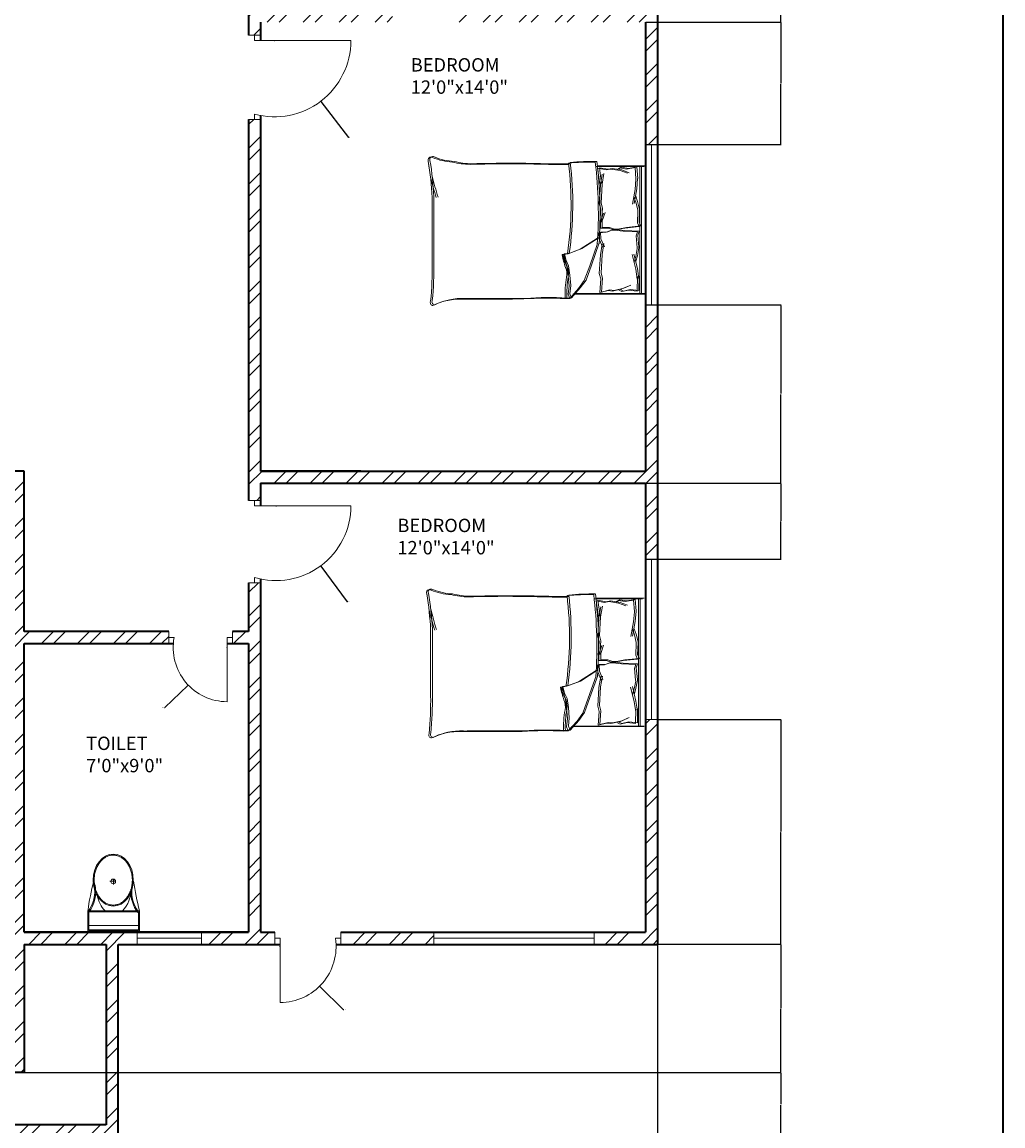
# Model space of a CAD drawing. Units: inches. Extents: x 392 to 1254, y 1207 to 2665.
# Tile 4 of 15: x 887 to 1254, y 1414 to 1827. Entities that reach past the tile are written whole.
import ezdxf

# ---------------------------------------------------------------- set-up
doc = ezdxf.new("R2010")
doc.units = ezdxf.units.IN
for name, color, linetype, lineweight in [('A-ANNO-DIMS', 2, 'Continuous', 18), ('A-ANNO-TTLB', 7, 'Continuous', 35), ('A-AREA-IDEN', 7, 'Continuous', 18), ('A-DOOR', 3, 'Continuous', 18), ('A-FLOR-FIXT', 9, 'Continuous', 18), ('A-FURN', 8, 'Continuous', 13), ('A-GLAZ', 4, 'Continuous', 18), ('A-WALL', 7, 'Continuous', 35), ('A-WALL-PATT', 252, 'Continuous', 13)]:
    doc.layers.add(name, color=color, linetype=linetype, lineweight=lineweight)
doc.styles.get("Standard").update_dxf_attribs({"font": 'arial.ttf'})
doc.dimstyles.get("Standard").update_dxf_attribs({"dimtxt": 0.18, "dimasz": 0.18, "dimexe": 0.18, "dimexo": 0.0625, "dimgap": 0.09, "dimtad": 0, "dimtih": 1, "dimtoh": 1, "dimdec": 4, "dimzin": 0, "dimdsep": 46, "dimtxsty": 'Standard', "dimcen": 0.09, "dimadec": 0, "dimazin": 0, "dimtfac": 1, "dimtdec": 4, "dimtofl": 0, "dimtmove": 0, "dimatfit": 3, "dimfxl": 1, "dimtolj": 1, "dimtzin": 0, "dimarcsym": 0})

# ---------------------------------------------------------------- blocks, each defined once
blk = doc.blocks.new('A$C31115884')
for p, q in [((283, 498), (223, 498)), ((258, 466), (258, 523)), ((0, 200), (0, 0)), ((520, 200), (0, 200)), ((10, 190), (10, 10)), ((510, 190), (10, 190)), ((510, 10), (510, 190)), ((520, 0), (520, 200)), ((510, 54), (0, 54)), ((10, 10), (510, 10)), ((0, 0), (520, 0))]:
    blk.add_line(p, q)
blk.add_circle((256, 496), 23.6)
for centre, radius, start, end in [((2778, -205), 2807, 165.4549, 171.7133), ((-295, 403), 365, 324.2091, 9.3499), ((-295, 403), 375, 324.2091, 9.3499), ((806, 403), 365, 170.6501, 215.7909), ((3237, 905), 2807, 188.2867, 194.5451), ((384, 406), 293, 190.2774, 224.1564), ((139, 406), 293, 315.8436, 2.6563), ((806, 403), 375, 179.2036, 215.7909)]:
    blk.add_arc(centre, radius, start, end)
blk.add_ellipse((256, 510), major_axis=(0, -261), ratio=0.772727)
blk.add_open_spline([(256, 259), (263, 259), (270, 260), (288, 262), (299, 265), (320, 273), (330, 278), (350, 291), (360, 299), (378, 316), (386, 326), (402, 347), (409, 358), (421, 383), (427, 395), (436, 422), (440, 436), (445, 465), (447, 480), (448, 509), (448, 524), (445, 553), (443, 568), (436, 596), (432, 610), (422, 636), (416, 649), (402, 672), (395, 683), (379, 703), (370, 712), (351, 728), (341, 735), (321, 746), (310, 751), (289, 757), (278, 759), (256, 761), (245, 761), (223, 757), (212, 754), (191, 746), (181, 741), (161, 728), (151, 720), (133, 703), (125, 693), (110, 672), (103, 660), (90, 636), (85, 623), (76, 596), (72, 582), (67, 553), (66, 538), (64, 509), (65, 494), (68, 465), (70, 450), (77, 422), (81, 408), (91, 382), (97, 370), (111, 346), (118, 335), (135, 316), (144, 307), (162, 291), (172, 284), (193, 273), (203, 269), (225, 262), (236, 260), (250, 259), (253, 259), (256, 259)], degree=3, knots=[0, 0, 0, 0, 0.110105, 0.110105, 0.285049, 0.285049, 0.459994, 0.459994, 0.634938, 0.634938, 0.809882, 0.809882, 0.984827, 0.984827, 1.159771, 1.159771, 1.334715, 1.334715, 1.50966, 1.50966, 1.684604, 1.684604, 1.859549, 1.859549, 2.034493, 2.034493, 2.209437, 2.209437, 2.384382, 2.384382, 2.559326, 2.559326, 2.73427, 2.73427, 2.909215, 2.909215, 3.084159, 3.084159, 3.259103, 3.259103, 3.434048, 3.434048, 3.608992, 3.608992, 3.783936, 3.783936, 3.958881, 3.958881, 4.133825, 4.133825, 4.30877, 4.30877, 4.483714, 4.483714, 4.658658, 4.658658, 4.833603, 4.833603, 5.008547, 5.008547, 5.183491, 5.183491, 5.358436, 5.358436, 5.53338, 5.53338, 5.708324, 5.708324, 5.883269, 5.883269, 6.058213, 6.058213, 6.233158, 6.233158, 6.283185, 6.283185, 6.283185, 6.283185])
blk = doc.blocks.new('BED-DOUBLE')
for p, q in [((3.47, 63.33), (3.47, 81.44)), ((3.47, 79.91), (51.27, 79.91)), ((3.48, 63.33), (3.48, 81.44)), ((3.48, 79.91), (51.27, 79.91)), ((3.7, 62.69), (3.7, 80.8)), ((3.7, 62.69), (3.7, 80.8)), ((3.7, 79.27), (51.49, 79.27)), ((3.7, 79.27), (51.49, 79.27)), ((16.88, 78.42), (19.77, 79.14)), ((16.88, 78.42), (19.77, 79.14)), ((17.11, 77.78), (20, 78.5)), ((17.11, 77.78), (20, 78.5)), ((19.77, 79.14), (20.09, 79.14)), ((19.77, 79.14), (20.09, 79.14)), ((20, 78.5), (20.32, 78.5)), ((20, 78.5), (20.32, 78.5)), ((20.09, 79.14), (24.54, 78.99)), ((20.09, 79.14), (24.54, 78.99)), ((20.32, 78.5), (24.77, 78.35)), ((20.32, 78.5), (24.77, 78.35)), ((24.54, 78.99), (25.98, 79.57)), ((24.54, 78.99), (25.98, 79.57)), ((24.77, 78.35), (26.21, 78.93)), ((24.77, 78.35), (26.21, 78.93)), ((25.98, 79.57), (26.56, 74.22)), ((25.98, 79.57), (26.56, 74.22)), ((26.21, 78.93), (26.79, 73.58)), ((26.21, 78.93), (26.79, 73.58)), ((27.98, 78.95), (27.73, 73.58)), ((27.98, 78.95), (27.73, 73.58)), ((29.46, 78.46), (27.98, 78.95)), ((29.46, 78.46), (27.98, 78.95)), ((33.88, 78.89), (29.46, 78.46)), ((33.88, 78.89), (29.46, 78.46)), ((34.2, 78.91), (33.88, 78.89)), ((34.2, 78.91), (33.88, 78.89)), ((37.14, 78.36), (34.2, 78.91)), ((37.14, 78.36), (34.2, 78.91)), ((45.71, 78.9), (41.91, 78.37)), ((45.71, 78.9), (41.91, 78.37)), ((50.11, 78.89), (44.71, 78.98)), ((44.71, 78.98), (45.71, 78.9)), ((50.11, 78.89), (44.71, 78.98)), ((44.71, 78.98), (45.71, 78.9)), ((50.11, 78.89), (49.73, 75.67)), ((50.11, 78.89), (49.73, 75.67)), ((51.27, 81.44), (51.27, 54.83)), ((51.27, 81.44), (51.27, 54.83)), ((51.49, 81.44), (51.49, 80.8)), ((51.49, 80.8), (51.49, 54.19)), ((51.49, 80.8), (51.49, 54.19)), ((3.89, 78.13), (4.47, 74.95)), ((3.89, 78.13), (4.47, 74.95)), ((3.9, 78.1), (8.18, 78.43)), ((3.9, 78.1), (8.18, 78.43)), ((4.47, 74.95), (4.04, 72.34)), ((4.47, 74.95), (4.04, 72.34)), ((4.12, 77.49), (4.7, 74.31)), ((4.12, 77.49), (4.7, 74.31)), ((4.13, 77.47), (8.41, 77.79)), ((4.13, 77.47), (8.41, 77.79)), ((5.05, 72.49), (6.06, 75.23)), ((5.05, 72.49), (6.06, 75.23)), ((5.28, 71.85), (6.29, 74.6)), ((5.28, 71.85), (6.29, 74.6)), ((8.18, 78.43), (8.28, 78.42)), ((8.18, 78.43), (8.28, 78.42)), ((8.28, 78.42), (12.11, 78.13)), ((8.28, 78.42), (12.11, 78.13)), ((8.41, 77.79), (8.51, 77.78)), ((8.41, 77.79), (8.51, 77.78)), ((8.51, 77.78), (12.34, 77.49)), ((8.51, 77.78), (12.34, 77.49)), ((12.11, 78.13), (17.6, 77.11)), ((12.11, 78.13), (17.6, 77.11)), ((12.34, 77.49), (17.83, 76.48)), ((12.34, 77.49), (17.83, 76.48)), ((14.85, 77.69), (16.88, 78.42)), ((14.85, 77.69), (16.88, 78.42)), ((15.08, 77.05), (17.11, 77.78)), ((15.08, 77.05), (17.11, 77.78)), ((28.21, 78.31), (27.96, 72.94)), ((28.21, 78.31), (27.96, 72.94)), ((29.68, 77.82), (28.21, 78.31)), ((29.68, 77.82), (28.21, 78.31)), ((34.11, 78.25), (29.68, 77.82)), ((34.11, 78.25), (29.68, 77.82)), ((34.43, 78.27), (34.11, 78.25)), ((34.43, 78.27), (34.11, 78.25)), ((37.36, 77.73), (34.43, 78.27)), ((37.36, 77.73), (34.43, 78.27)), ((41.91, 78.37), (36.49, 77.02)), ((41.91, 78.37), (36.5, 77.02)), ((42.14, 77.73), (36.72, 76.38)), ((42.14, 77.73), (36.72, 76.38)), ((39.2, 77.77), (37.14, 78.36)), ((39.2, 77.77), (37.14, 78.36)), ((39.43, 77.13), (37.36, 77.73)), ((39.43, 77.13), (37.36, 77.73)), ((45.94, 78.26), (42.14, 77.73)), ((45.94, 78.26), (42.14, 77.73)), ((50.34, 78.25), (44.94, 78.34)), ((44.94, 78.34), (45.94, 78.26)), ((50.34, 78.25), (44.94, 78.34)), ((44.94, 78.34), (45.94, 78.26)), ((49.31, 73.19), (48.13, 75.86)), ((49.31, 73.19), (48.13, 75.86)), ((49.54, 72.55), (48.36, 75.22)), ((49.54, 72.55), (48.36, 75.22)), ((49.73, 75.67), (50.33, 73.1)), ((49.73, 75.67), (50.33, 73.1)), ((50.34, 78.25), (49.96, 75.04)), ((50.34, 78.25), (49.96, 75.04)), ((49.96, 75.04), (50.56, 72.47)), ((49.96, 75.04), (50.56, 72.47)), ((4.04, 72.34), (4.62, 71.33)), ((4.04, 72.34), (4.62, 71.33)), ((4.7, 74.31), (4.27, 71.7)), ((4.7, 74.31), (4.27, 71.7)), ((4.27, 71.7), (4.85, 70.69)), ((4.27, 71.7), (4.85, 70.69)), ((4.47, 68.87), (5.05, 72.49)), ((4.47, 68.87), (5.05, 72.49)), ((4.7, 68.23), (5.28, 71.85)), ((4.7, 68.23), (5.28, 71.85)), ((26.56, 74.22), (27.14, 71.04)), ((26.56, 74.22), (27.14, 71.04)), ((26.79, 73.58), (27.37, 70.4)), ((26.79, 73.58), (27.37, 70.4)), ((27.14, 71.04), (27.14, 69.74)), ((27.14, 71.04), (27.14, 69.74)), ((27.73, 73.58), (27.35, 70.36)), ((27.73, 73.58), (27.35, 70.36)), ((27.35, 70.36), (27.44, 69.07)), ((27.35, 70.36), (27.44, 69.07)), ((27.37, 70.4), (27.37, 69.1)), ((27.37, 70.4), (27.37, 69.1)), ((27.96, 72.94), (27.58, 69.73)), ((27.96, 72.94), (27.58, 69.73)), ((50.11, 69.61), (49.31, 73.19)), ((50.11, 69.61), (49.31, 73.19)), ((50.34, 68.97), (49.54, 72.55)), ((50.34, 68.97), (49.54, 72.55)), ((50.33, 73.1), (49.81, 72.06)), ((50.33, 73.1), (49.81, 72.06)), ((50.56, 72.47), (50.04, 71.42)), ((50.56, 72.47), (50.04, 71.42)), ((4.18, 64.1), (4.76, 67.28)), ((4.18, 64.1), (4.76, 67.28)), ((4.41, 63.46), (4.99, 66.64)), ((4.41, 63.46), (4.99, 66.64)), ((4.76, 67.28), (4.47, 68.87)), ((4.76, 67.28), (4.47, 68.87)), ((4.99, 66.64), (4.7, 68.23)), ((4.99, 66.64), (4.7, 68.23)), ((24.1, 65.18), (20.96, 66.27)), ((24.1, 65.18), (20.96, 66.27)), ((27.14, 69.74), (26.56, 67.86)), ((27.14, 69.74), (26.56, 67.86)), ((26.56, 67.86), (26.56, 65.18)), ((26.56, 67.86), (26.56, 65.18)), ((27.37, 69.1), (26.79, 67.22)), ((27.37, 69.1), (26.79, 67.22)), ((26.79, 67.22), (26.79, 64.54)), ((26.79, 67.22), (26.79, 64.54)), ((27.44, 69.07), (28.13, 67.23)), ((27.44, 69.07), (28.13, 67.23)), ((27.58, 69.73), (27.66, 68.43)), ((27.58, 69.73), (27.66, 68.43)), ((27.66, 68.43), (28.36, 66.59)), ((27.66, 68.43), (28.36, 66.59)), ((28.13, 67.23), (28.3, 64.55)), ((28.13, 67.23), (28.3, 64.55)), ((28.36, 66.59), (28.53, 63.91)), ((28.36, 66.59), (28.53, 63.91)), ((49.92, 68.01), (50.11, 69.61)), ((49.92, 68.01), (50.11, 69.61)), ((50.7, 64.87), (49.92, 68.01)), ((50.7, 64.87), (49.92, 68.01)), ((50.15, 67.37), (50.34, 68.97)), ((50.15, 67.37), (50.34, 68.97)), ((50.93, 64.23), (50.15, 67.37)), ((50.93, 64.23), (50.15, 67.37)), ((9.28, 64.82), (4.18, 64.1)), ((9.28, 64.82), (4.18, 64.1)), ((9.51, 64.19), (4.41, 63.46)), ((9.51, 64.19), (4.41, 63.46)), ((6.38, 65.81), (10.41, 65.15)), ((6.38, 65.81), (10.41, 65.15)), ((6.61, 65.17), (10.64, 64.51)), ((6.61, 65.17), (10.64, 64.51)), ((10.41, 65.15), (9.28, 64.82)), ((10.41, 65.15), (9.28, 64.82)), ((10.64, 64.51), (9.51, 64.19)), ((10.64, 64.51), (9.51, 64.19)), ((10.41, 65.15), (17.42, 64.72)), ((10.41, 65.15), (17.42, 64.72)), ((10.64, 64.51), (17.65, 64.08)), ((10.64, 64.51), (17.65, 64.08)), ((17.42, 64.72), (19.38, 65.27)), ((17.42, 64.72), (19.38, 65.27)), ((17.65, 64.08), (19.61, 64.63)), ((17.65, 64.08), (19.61, 64.63)), ((19.38, 65.27), (24.52, 64.87)), ((19.38, 65.27), (24.52, 64.87)), ((19.61, 64.63), (24.74, 64.23)), ((19.61, 64.63), (24.74, 64.23)), ((24.33, 64.54), (21.19, 65.63)), ((24.33, 64.54), (21.19, 65.63)), ((26.56, 65.18), (24.1, 65.18)), ((26.56, 65.18), (24.1, 65.18)), ((26.79, 64.54), (24.33, 64.54)), ((26.79, 64.54), (24.33, 64.54)), ((28.3, 64.55), (30.75, 64.7)), ((28.3, 64.55), (30.75, 64.7)), ((28.53, 63.91), (30.98, 64.06)), ((28.53, 63.91), (30.98, 64.06)), ((30.26, 64.06), (34.45, 57.57)), ((30.26, 64.06), (34.45, 57.57)), ((30.49, 63.42), (34.68, 56.93)), ((30.49, 63.42), (34.68, 56.93)), ((30.75, 64.7), (33.82, 65.99)), ((30.75, 64.7), (33.82, 65.99)), ((30.98, 64.06), (34.05, 65.35)), ((30.98, 64.06), (34.05, 65.35)), ((40.64, 61.13), (32.31, 64.06)), ((40.64, 61.13), (32.31, 64.06)), ((40.87, 60.49), (32.53, 63.42)), ((40.87, 60.49), (32.53, 63.42)), ((32.56, 65.81), (36.6, 65.15)), ((32.56, 65.81), (36.6, 65.15)), ((32.79, 65.17), (36.82, 64.51)), ((32.79, 65.17), (36.82, 64.51)), ((36.6, 65.15), (43.61, 64.72)), ((36.6, 65.15), (43.61, 64.72)), ((36.82, 64.51), (43.83, 64.08)), ((36.82, 64.51), (43.83, 64.08)), ((43.61, 64.72), (45.57, 65.27)), ((43.61, 64.72), (45.57, 65.27)), ((43.83, 64.08), (45.79, 64.63)), ((43.83, 64.08), (45.79, 64.63)), ((45.57, 65.27), (50.7, 64.87)), ((45.57, 65.27), (50.7, 64.87)), ((45.79, 64.63), (50.93, 64.23)), ((45.79, 64.63), (50.93, 64.23)), ((46.22, 59.11), (40.64, 61.13)), ((46.22, 59.11), (40.64, 61.13)), ((46.45, 58.47), (40.87, 60.49)), ((46.45, 58.47), (40.87, 60.49)), ((49.16, 56.95), (46.22, 59.11)), ((49.16, 56.95), (46.22, 59.11)), ((49.39, 56.31), (46.45, 58.47)), ((49.39, 56.31), (46.45, 58.47)), ((34.45, 57.57), (36.15, 53.08)), ((34.45, 57.57), (36.15, 53.08)), ((34.68, 56.93), (36.38, 52.44)), ((34.68, 56.93), (36.38, 52.44)), ((52.87, 53.7), (49.16, 56.95)), ((52.87, 53.7), (49.16, 56.95)), ((53.1, 53.06), (49.39, 56.31)), ((53.1, 53.06), (49.39, 56.31)), ((51.33, 53.08), (52.87, 53.7)), ((51.33, 53.08), (52.87, 53.7)), ((52.95, 51.95), (52.87, 53.7, 3.87)), ((52.95, 51.95), (52.87, 53.7, 3.87)), ((36.15, 53.08), (36.46, 51.07)), ((36.15, 53.08), (36.46, 51.07)), ((36.38, 52.44), (36.69, 50.43)), ((36.38, 52.44), (36.69, 50.43)), ((36.46, 51.07), (38.94, 51.68)), ((36.46, 51.07), (38.94, 51.68)), ((36.69, 50.43), (39.17, 51.05)), ((36.69, 50.43), (39.17, 51.05)), ((38.94, 51.68), (40.95, 52.61)), ((38.94, 51.68), (40.95, 52.61)), ((39.17, 51.05), (41.18, 51.97)), ((39.17, 51.05), (41.18, 51.97)), ((40.95, 52.61), (44.36, 53.08)), ((40.95, 52.61), (44.36, 53.08)), ((41.18, 51.97), (44.59, 52.44)), ((41.18, 51.97), (44.59, 52.44)), ((44.36, 53.08), (48.23, 53.39)), ((44.36, 53.08), (48.23, 53.39)), ((44.59, 52.44), (48.46, 52.75)), ((44.59, 52.44), (48.46, 52.75)), ((48.23, 53.39), (51.33, 53.08)), ((48.23, 53.39), (51.33, 53.08)), ((48.46, 52.75), (51.56, 52.44)), ((48.46, 52.75), (51.56, 52.44)), ((51.56, 52.44), (53.1, 53.06)), ((51.56, 52.44), (53.1, 53.06)), ((53.18, 51.31), (53.1, 53.06, 3.87)), ((53.18, 51.31), (53.1, 53.06, 3.87)), ((15.06, 2.2), (39.68, 2.2)), ((15.06, 2.2), (39.68, 2.2)), ((15.29, 1.56), (39.91, 1.56)), ((15.29, 1.56), (39.91, 1.56))]:
    blk.add_line(p, q)
for centre, radius, start, end in [((85.16, 61.35), 83.31, 178.7218, 185.604), ((85.16, 61.35), 83.31, 178.7218, 185.604), ((21.36, -100.61), 164.97, 86.0865, 96.7821), ((21.36, -100.61), 164.97, 86.0865, 96.7821), ((85.39, 60.71), 83.31, 178.7218, 185.604), ((85.39, 60.71), 83.31, 178.7218, 185.604), ((21.59, -101.25), 164.97, 86.0865, 96.7821), ((21.59, -101.25), 164.97, 86.0865, 96.7821), ((17.76, -74.87), 129.02, 81.7845, 96.9006), ((17.76, -74.87), 129.02, 81.7845, 96.9006), ((17.98, -75.51), 129.02, 81.7845, 96.9006), ((17.98, -75.51), 129.02, 81.7845, 96.9006), ((-167.31, 50.27), 170.11, 358.4762, 1.0082), ((-167.31, 50.27), 170.11, 358.4762, 1.0082), ((-167.08, 49.63), 170.11, 358.4762, 1.0082), ((-167.08, 49.63), 170.11, 358.4762, 1.0082), ((36.64, 51), 0.185, 160.2464, 271.1377), ((36.64, 51), 0.185, 160.2464, 271.1377), ((31.15, 79.96), 29.65, 280.6617, 289.8806), ((31.15, 79.96), 29.65, 280.6617, 289.8806), ((36.86, 50.36), 0.185, 160.2464, 271.1377), ((36.86, 50.36), 0.185, 160.2464, 271.1377), ((31.38, 79.32), 29.65, 280.6617, 289.8806), ((31.38, 79.32), 29.65, 280.6617, 289.8806), ((43.74, 46.38), 6.22, 78.6608, 113.7384), ((43.74, 46.38), 6.22, 78.6608, 113.7384), ((43.97, 45.74), 6.22, 78.6608, 113.7384), ((43.97, 45.74), 6.22, 78.6608, 113.7384), ((51.33, 88.1), 36.18, 259.8763, 272.5657), ((51.33, 88.1), 36.18, 259.8763, 272.5657), ((51.56, 87.46), 36.18, 259.8763, 272.5657), ((51.56, 87.46), 36.18, 259.8763, 272.5657), ((182.27, 45.13), 129.5, 176.9791, 183.8365), ((182.27, 45.13), 129.5, 176.9791, 183.8365), ((182.49, 44.49), 129.5, 176.9791, 183.8365), ((182.49, 44.49), 129.5, 176.9791, 183.8365), ((484.82, 30.83), 482.31, 178.2277, 181.7185), ((484.82, 30.83), 482.31, 178.2277, 181.7185), ((485.05, 30.19), 482.31, 178.2277, 181.7185), ((485.05, 30.19), 482.31, 178.2277, 181.7185), ((-4508.74, 13.62), 4561.86, 0.00217, 0.28689), ((-4508.74, 13.62), 4561.86, 0.00217, 0.28689), ((-4508.51, 12.98), 4561.86, 0.00217, 0.28689), ((-4508.52, 12.98), 4561.86, 0.00217, 0.28689), ((-26.9, 16.93), 29.63, 346.0648, 358.9113), ((-26.9, 16.93), 29.63, 346.0648, 358.9113), ((-26.67, 16.29), 29.63, 346.0648, 358.9113), ((-26.67, 16.29), 29.63, 346.0648, 358.9113), ((76.16, 12.78), 23.07, 177.4714, 206.4681), ((76.16, 12.78), 23.07, 177.4714, 206.4681), ((76.39, 12.14), 23.07, 177.4714, 206.4681), ((76.39, 12.14), 23.07, 177.4714, 206.4681), ((-21.66, 11.17), 23.56, 337.9751, 356.652), ((-21.66, 11.17), 23.56, 337.9751, 356.652), ((-21.43, 10.53), 23.56, 337.9751, 356.652), ((-21.43, 10.53), 23.56, 337.9751, 356.652), ((1.09, 1.72), 1.09, 146.1736, 293.4781), ((1.09, 1.72), 1.09, 146.1736, 293.4781), ((1.32, 1.09), 1.09, 146.1736, 293.4781), ((1.32, 1.09), 1.09, 146.1736, 293.4781), ((21.43, -119.39), 121.76, 92.9958, 99.4091), ((21.43, -119.39), 121.76, 92.9958, 99.4091), ((21.66, -120.03), 121.76, 92.9958, 99.4091), ((21.65, -120.03), 121.76, 92.9958, 99.4091), ((-17.22, 105.15), 106.46, 283.3832, 287.7053), ((-17.22, 105.15), 106.46, 283.3832, 287.7053), ((-16.99, 104.52), 106.46, 283.3832, 287.7053), ((-16.99, 104.52), 106.46, 283.3832, 287.7053), ((41.15, -130.83), 133.04, 84.4998, 90.6351), ((41.15, -130.83), 133.04, 84.4998, 90.6351), ((41.38, -131.47), 133.04, 84.4998, 90.6351), ((41.38, -131.47), 133.04, 84.4998, 90.6351), ((54.41, 2.57), 1.1, 242.6588, 356.02), ((54.41, 2.57), 1.1, 242.6588, 356.02), ((54.64, 1.93), 1.1, 242.6588, 356.02), ((54.64, 1.93), 1.1, 242.6588, 356.02)]:
    blk.add_arc(centre, radius, start, end)
blk = doc.blocks.new('WIN-60-A')
for p, q in [((0, 60), (4.5, 60)), ((4.5, 60), (2.25, 60)), ((2.25, 60), (2.25, 0)), ((2.25, 0), (0, 0)), ((0, 0), (4.5, 0))]:
    blk.add_line(p, q)
blk = doc.blocks.new('WIN-24-A')
for p, q in [((0, 0), (0, 4.5)), ((0, 4.5), (0, 2.25)), ((24, 2.25), (24, 4.5)), ((24, 4.5), (24, 0)), ((0, 2.25), (24, 2.25))]:
    blk.add_line(p, q)
blk = doc.blocks.new('*D25')
at = {"layer": 'A-ANNO-DIMS', "color": 0, "lineweight": -2, "transparency": 16777216}
for p, q in [((541.28, 1482.23), (541.28, 1364.02)), ((1124.78, 1482.23), (1124.78, 1364.02)), ((541.46, 1364.2), (832.64, 1364.2)), ((1124.6, 1364.2), (833.43, 1364.2))]:
    blk.add_line(p, q, dxfattribs=at)
at = {"layer": 'A-ANNO-DIMS', "color": 0, "transparency": 16777216}
for points in [[(541.46, 1364.23), (541.46, 1364.17), (541.28, 1364.2)], [(1124.6, 1364.23), (1124.6, 1364.17), (1124.78, 1364.2)]]:
    blk.add_solid(points, dxfattribs=at)
at = {"layer": 'Defpoints', "color": 0, "transparency": 16777216}
for p in [(541.28, 1482.3), (1124.78, 1482.3), (1124.78, 1364.2)]:
    blk.add_point(p, dxfattribs=at)
at = {"layer": 'A-ANNO-DIMS', "color": 0, "transparency": 16777216, "insert": (833.03, 1364.2), "char_height": 0.18, "attachment_point": 5}
blk.add_mtext('\\A1;583.5', dxfattribs=at)
blk = doc.blocks.new('*D27')
at = {"layer": 'A-ANNO-DIMS', "color": 0, "lineweight": -2, "transparency": 16777216}
for p, q in [((1124.84, 1482.3), (1171.06, 1482.3)), ((1170.88, 1482.12), (1170.88, 1458.48)), ((1170.88, 1434.48), (1170.88, 1458.11)), ((887.84, 1434.3), (1171.06, 1434.3))]:
    blk.add_line(p, q, dxfattribs=at)
at = {"layer": 'A-ANNO-DIMS', "color": 0, "transparency": 16777216}
for points in [[(1170.85, 1482.12), (1170.91, 1482.12), (1170.88, 1482.3)], [(1170.85, 1434.48), (1170.91, 1434.48), (1170.88, 1434.3)]]:
    blk.add_solid(points, dxfattribs=at)
at = {"layer": 'Defpoints', "color": 0, "transparency": 16777216}
for p in [(1124.78, 1482.3), (1170.88, 1482.3), (887.78, 1434.3)]:
    blk.add_point(p, dxfattribs=at)
at = {"layer": 'A-ANNO-DIMS', "color": 0, "transparency": 16777216, "insert": (1170.88, 1458.3), "char_height": 0.18, "attachment_point": 5}
blk.add_mtext('\\A1;48', dxfattribs=at)
blk = doc.blocks.new('*D30')
at = {"layer": 'A-ANNO-DIMS', "color": 0, "lineweight": -2, "transparency": 16777216}
for p, q in [((1124.84, 1566.38), (1171.06, 1566.38)), ((1170.88, 1566.2), (1170.88, 1524.52)), ((1170.88, 1482.48), (1170.88, 1524.16)), ((1124.84, 1482.3), (1171.06, 1482.3))]:
    blk.add_line(p, q, dxfattribs=at)
at = {"layer": 'A-ANNO-DIMS', "color": 0, "transparency": 16777216}
for points in [[(1170.85, 1566.2), (1170.91, 1566.2), (1170.88, 1566.38)], [(1170.85, 1482.48), (1170.91, 1482.48), (1170.88, 1482.3)]]:
    blk.add_solid(points, dxfattribs=at)
at = {"layer": 'Defpoints', "color": 0, "transparency": 16777216}
for p in [(1124.78, 1566.38), (1170.88, 1566.38), (1124.78, 1482.3)]:
    blk.add_point(p, dxfattribs=at)
at = {"layer": 'A-ANNO-DIMS', "color": 0, "transparency": 16777216, "insert": (1170.88, 1524.34), "char_height": 0.18, "attachment_point": 5}
blk.add_mtext('\\A1;84.09', dxfattribs=at)
blk = doc.blocks.new('*D31')
at = {"layer": 'A-ANNO-DIMS', "color": 0, "lineweight": -2, "transparency": 16777216}
for p, q in [((1120.34, 1721.46), (1171.06, 1721.46)), ((1170.88, 1721.28), (1170.88, 1688.31)), ((1170.88, 1654.98), (1170.88, 1687.94)), ((1120.34, 1654.8), (1171.06, 1654.8))]:
    blk.add_line(p, q, dxfattribs=at)
at = {"layer": 'A-ANNO-DIMS', "color": 0, "transparency": 16777216}
for points in [[(1170.85, 1721.28), (1170.91, 1721.28), (1170.88, 1721.46)], [(1170.85, 1654.98), (1170.91, 1654.98), (1170.88, 1654.8)]]:
    blk.add_solid(points, dxfattribs=at)
at = {"layer": 'Defpoints', "color": 0, "transparency": 16777216}
for p in [(1120.28, 1721.46), (1170.88, 1721.46), (1120.28, 1654.8)]:
    blk.add_point(p, dxfattribs=at)
at = {"layer": 'A-ANNO-DIMS', "color": 0, "transparency": 16777216, "insert": (1170.88, 1688.13), "char_height": 0.18, "attachment_point": 5}
blk.add_mtext('\\A1;66.66', dxfattribs=at)
blk = doc.blocks.new('*D32')
at = {"layer": 'A-ANNO-DIMS', "color": 0, "lineweight": -2, "transparency": 16777216}
for p, q in [((1120.34, 1842.92), (1171.06, 1842.92)), ((1170.88, 1842.74), (1170.88, 1835.29)), ((1170.88, 1827.48), (1170.88, 1834.93)), ((1120.34, 1827.3), (1171.06, 1827.3))]:
    blk.add_line(p, q, dxfattribs=at)
at = {"layer": 'A-ANNO-DIMS', "color": 0, "transparency": 16777216}
for points in [[(1170.85, 1842.74), (1170.91, 1842.74), (1170.88, 1842.92)], [(1170.85, 1827.48), (1170.91, 1827.48), (1170.88, 1827.3)]]:
    blk.add_solid(points, dxfattribs=at)
at = {"layer": 'Defpoints', "color": 0, "transparency": 16777216}
for p in [(1120.28, 1842.92), (1170.88, 1842.92), (1120.28, 1827.3)]:
    blk.add_point(p, dxfattribs=at)
at = {"layer": 'A-ANNO-DIMS', "color": 0, "transparency": 16777216, "insert": (1170.88, 1835.11), "char_height": 0.18, "attachment_point": 5}
blk.add_mtext('\\A1;15.624', dxfattribs=at)
blk = doc.blocks.new('*D42')
at = {"layer": 'A-ANNO-DIMS', "color": 0, "lineweight": -2, "transparency": 16777216}
for p, q in [((1120.34, 1827.3), (1171.06, 1827.3)), ((1170.88, 1827.12), (1170.88, 1804.56)), ((1170.88, 1781.64), (1170.88, 1804.19)), ((1120.34, 1781.46), (1171.06, 1781.46))]:
    blk.add_line(p, q, dxfattribs=at)
at = {"layer": 'A-ANNO-DIMS', "color": 0, "transparency": 16777216}
for points in [[(1170.85, 1827.12), (1170.91, 1827.12), (1170.88, 1827.3)], [(1170.85, 1781.64), (1170.91, 1781.64), (1170.88, 1781.46)]]:
    blk.add_solid(points, dxfattribs=at)
at = {"layer": 'Defpoints', "color": 0, "transparency": 16777216}
for p in [(1120.28, 1827.3), (1120.28, 1781.46), (1170.88, 1781.46)]:
    blk.add_point(p, dxfattribs=at)
at = {"layer": 'A-ANNO-DIMS', "color": 0, "transparency": 16777216, "insert": (1170.88, 1804.38), "char_height": 0.18, "attachment_point": 5}
blk.add_mtext('\\A1;45.84', dxfattribs=at)
blk = doc.blocks.new('*D43')
at = {"layer": 'A-ANNO-DIMS', "color": 0, "lineweight": -2, "transparency": 16777216}
for p, q in [((1120.34, 1654.8), (1171.06, 1654.8)), ((1170.88, 1654.62), (1170.88, 1640.77)), ((1170.88, 1626.56), (1170.88, 1640.41)), ((1120.34, 1626.38), (1171.06, 1626.38))]:
    blk.add_line(p, q, dxfattribs=at)
at = {"layer": 'A-ANNO-DIMS', "color": 0, "transparency": 16777216}
for points in [[(1170.85, 1654.62), (1170.91, 1654.62), (1170.88, 1654.8)], [(1170.85, 1626.56), (1170.91, 1626.56), (1170.88, 1626.38)]]:
    blk.add_solid(points, dxfattribs=at)
at = {"layer": 'Defpoints', "color": 0, "transparency": 16777216}
for p in [(1120.28, 1654.8), (1120.28, 1626.38), (1170.88, 1626.38)]:
    blk.add_point(p, dxfattribs=at)
at = {"layer": 'A-ANNO-DIMS', "color": 0, "transparency": 16777216, "insert": (1170.88, 1640.59), "char_height": 0.18, "attachment_point": 5}
blk.add_mtext('\\A1;28.415', dxfattribs=at)
blk = doc.blocks.new('*D51')
at = {"layer": 'A-ANNO-DIMS', "color": 0, "lineweight": -2, "transparency": 16777216}
for p, q in [((887.84, 1434.3), (1171.06, 1434.3)), ((1170.88, 1434.12), (1170.88, 1422.48)), ((1170.88, 1410.48), (1170.88, 1422.11)), ((923.05, 1410.3), (1171.06, 1410.3))]:
    blk.add_line(p, q, dxfattribs=at)
at = {"layer": 'A-ANNO-DIMS', "color": 0, "transparency": 16777216}
for points in [[(1170.85, 1434.12), (1170.91, 1434.12), (1170.88, 1434.3)], [(1170.85, 1410.48), (1170.91, 1410.48), (1170.88, 1410.3)]]:
    blk.add_solid(points, dxfattribs=at)
at = {"layer": 'Defpoints', "color": 0, "transparency": 16777216}
for p in [(887.78, 1434.3), (922.99, 1410.3), (1170.88, 1410.3)]:
    blk.add_point(p, dxfattribs=at)
at = {"layer": 'A-ANNO-DIMS', "color": 0, "transparency": 16777216, "insert": (1170.88, 1422.3), "char_height": 0.18, "attachment_point": 5}
blk.add_mtext('\\A1;24', dxfattribs=at)
blk = doc.blocks.new('*D90')
at = {"layer": 'A-ANNO-DIMS', "color": 0, "lineweight": -2, "transparency": 16777216}
for p, q in [((981.43, 1820.38), (981.61, 1820.38)), ((981.52, 1820.29), (981.52, 1820.47)), ((1009.22, 1784.14), (998.94, 1797.59)), ((1009.4, 1784.14), (1009.22, 1784.14))]:
    blk.add_line(p, q, dxfattribs=at)
at = {"layer": 'A-ANNO-DIMS', "color": 0, "transparency": 16777216}
blk.add_solid([(998.96, 1797.6), (998.92, 1797.57), (998.83, 1797.73)], dxfattribs=at)
at = {"layer": 'Defpoints', "color": 0, "transparency": 16777216}
for p in [(981.52, 1820.38), (998.83, 1797.73)]:
    blk.add_point(p, dxfattribs=at)
at = {"layer": 'A-ANNO-DIMS', "color": 0, "transparency": 16777216, "insert": (1009.86, 1784.14), "char_height": 0.18, "attachment_point": 5}
blk.add_mtext('\\A1;R28.51', dxfattribs=at)
blk = doc.blocks.new('*D92')
at = {"layer": 'A-ANNO-DIMS', "color": 0, "lineweight": -2, "transparency": 16777216}
for p, q in [((981.98, 1646.33), (982.16, 1646.33)), ((982.07, 1646.24), (982.07, 1646.42)), ((1008.77, 1610.44), (998.87, 1623.75)), ((1008.95, 1610.44), (1008.77, 1610.44))]:
    blk.add_line(p, q, dxfattribs=at)
at = {"layer": 'A-ANNO-DIMS', "color": 0, "transparency": 16777216}
blk.add_solid([(998.89, 1623.77), (998.84, 1623.74), (998.76, 1623.9)], dxfattribs=at)
at = {"layer": 'Defpoints', "color": 0, "transparency": 16777216}
for p in [(982.07, 1646.33), (998.76, 1623.9)]:
    blk.add_point(p, dxfattribs=at)
at = {"layer": 'A-ANNO-DIMS', "color": 0, "transparency": 16777216, "insert": (1009.5, 1610.44), "char_height": 0.18, "attachment_point": 5}
blk.add_mtext('\\A1;R27.964', dxfattribs=at)
blk = doc.blocks.new('*D104')
at = {"layer": 'A-ANNO-DIMS', "color": 0, "lineweight": -2, "transparency": 16777216}
for p, q in [((963.71, 1593.29), (963.89, 1593.29)), ((963.8, 1593.2), (963.8, 1593.38)), ((940.47, 1570.83), (949.09, 1579.12)), ((940.29, 1570.83), (940.47, 1570.83))]:
    blk.add_line(p, q, dxfattribs=at)
at = {"layer": 'A-ANNO-DIMS', "color": 0, "transparency": 16777216}
blk.add_solid([(949.07, 1579.15), (949.11, 1579.1), (949.22, 1579.25)], dxfattribs=at)
at = {"layer": 'Defpoints', "color": 0, "transparency": 16777216}
for p in [(963.8, 1593.29), (949.22, 1579.25)]:
    blk.add_point(p, dxfattribs=at)
at = {"layer": 'A-ANNO-DIMS', "color": 0, "transparency": 16777216, "insert": (939.81, 1570.83), "char_height": 0.18, "attachment_point": 5}
blk.add_mtext('\\A1;R20.24', dxfattribs=at)
blk = doc.blocks.new('*D106')
at = {"layer": 'A-ANNO-DIMS', "color": 0, "lineweight": -2, "transparency": 16777216}
for p, q in [((983.48, 1481.48), (983.66, 1481.48)), ((983.57, 1481.39), (983.57, 1481.57)), ((1007.22, 1457.76), (998.48, 1466.52)), ((1007.4, 1457.76), (1007.22, 1457.76))]:
    blk.add_line(p, q, dxfattribs=at)
at = {"layer": 'A-ANNO-DIMS', "color": 0, "transparency": 16777216}
blk.add_solid([(998.5, 1466.55), (998.46, 1466.5), (998.35, 1466.65)], dxfattribs=at)
at = {"layer": 'Defpoints', "color": 0, "transparency": 16777216}
for p in [(983.57, 1481.48), (998.35, 1466.65)]:
    blk.add_point(p, dxfattribs=at)
at = {"layer": 'A-ANNO-DIMS', "color": 0, "transparency": 16777216, "insert": (1007.95, 1457.76), "char_height": 0.18, "attachment_point": 5}
blk.add_mtext('\\A1;R20.935', dxfattribs=at)

msp = doc.modelspace()

# ---------------------------------------------------------------- hatches: boundary and pattern name
at = {"layer": 'A-WALL-PATT'}
h = msp.add_hatch(dxfattribs=at)
h.set_pattern_fill('ANSI32', color=256)
h.paths.add_polyline_path([(579.5309, 2227.0453), (579.5309, 2229.2953), (541.2807, 2229.2953), (541.2807, 2182.3091), (545.7807, 2182.3091), (545.7807, 2224.7953), (579.5309, 2224.7953)])
h.paths.add_polyline_path([(655.4442, 2229.2953), (627.5309, 2229.2953), (627.5309, 2224.7953), (655.4442, 2224.7953), (655.4442, 2227.0453)])
h.paths.add_polyline_path([(703.0758, 2229.2953), (678.5257, 2229.2953), (678.5257, 2227.0453), (678.5257, 2224.7953), (689.7807, 2224.7953), (689.7807, 2158.6973), (694.2807, 2158.6973), (694.2807, 2224.7953), (703.0758, 2224.7953)])
h.paths.add_polyline_path([(768.5767, 2229.2953), (727.0758, 2229.2953), (727.0758, 2224.7953), (742.2807, 2224.7953), (742.2807, 2128.7953), (694.2807, 2128.7953), (694.2807, 2134.0554), (689.7807, 2134.0554), (689.7807, 2090.2854), (694.2807, 2090.2854), (694.2807, 2124.2953), (742.2807, 2124.2953), (742.2807, 2052.2953), (795.2124, 2052.2953), (795.2124, 2054.5453), (795.2124, 2056.7953), (746.7807, 2056.7953), (746.7807, 2224.7953), (768.5767, 2224.7953)])
h.paths.add_polyline_path([(867.5089, 2229.2953), (804.5767, 2229.2953), (804.5767, 2224.7953), (830.7807, 2224.7953), (830.7807, 2056.7953), (826.9066, 2056.7953), (826.9066, 2052.2953), (830.7807, 2052.2953), (830.7807, 1886.6777, -0.01766664), (830.8602, 1884.2953), (835.0818, 1884.2953, -0.04411348), (835.2807, 1889.9369), (835.2807, 2052.2953), (839.418, 2052.2953), (839.418, 2056.7953), (835.2807, 2056.7953), (835.2807, 2224.7953), (867.5089, 2224.7953)])
h.paths.add_polyline_path([(939.8604, 2229.2953), (903.5089, 2229.2953), (903.5089, 2227.0453), (903.5089, 2224.7953), (919.2807, 2224.7953), (919.2807, 2056.7953), (870.6499, 2056.7953), (870.6499, 2052.2953), (923.7807, 2052.2953), (923.7807, 2124.2953), (971.7807, 2124.2953), (971.7807, 2089.7112), (974.0307, 2089.7112), (976.2807, 2089.7112), (976.2807, 2133.56), (974.0307, 2133.56), (971.7807, 2133.56), (971.7807, 2128.7953), (923.7807, 2128.7953), (923.7807, 2224.7953), (939.8604, 2224.7953)])
h.paths.add_polyline_path([(1124.7807, 2229.2953), (1009.403, 2229.2953), (1009.403, 2224.7953), (1120.2807, 2224.7953), (1120.2807, 2184.7605), (1124.7807, 2184.7605)])
h.paths.add_polyline_path([(1124.7807, 2124.7605), (1120.2807, 2124.7605), (1120.2807, 2056.7953), (976.2807, 2056.7953), (976.2807, 2061.471), (971.7807, 2061.471), (971.7807, 2047.7483), (974.0307, 2047.7483), (976.2807, 2047.7483), (976.2807, 2052.2953), (1120.2807, 2052.2953), (1120.2807, 1992.457), (1124.7807, 1992.457)])
h.paths.add_polyline_path([(1124.7807, 1932.457), (1122.5307, 1932.457), (1120.2807, 1932.457), (1120.2807, 1884.2953), (976.2807, 1884.2953), (976.2807, 2019.9536), (971.7807, 2019.9536), (971.7807, 1884.2953), (869.0911, 1884.2953), (869.0911, 1879.7953), (971.7807, 1879.7953), (1013.7807, 1879.7953), (1013.7807, 1831.7953), (971.7807, 1831.7953), (971.7807, 1822.3831), (974.0307, 1822.3831), (976.2807, 1822.3831), (976.2807, 1827.2953), (1013.7807, 1827.2953), (1025.6191, 1827.2953), (1025.6191, 1829.5453), (1025.6191, 1831.7953), (1018.2807, 1831.7953), (1018.2807, 1879.7953), (1120.2807, 1879.7953), (1120.2807, 1866.9192), (1124.7807, 1866.9192)])
h.paths.add_polyline_path([(1124.7807, 1842.9192), (1122.5307, 1842.9192), (1120.2807, 1842.9192), (1120.2807, 1831.7953), (1050.2021, 1831.7953), (1050.2021, 1827.2953), (1120.2807, 1827.2953), (1120.2807, 1781.4559), (1124.7807, 1781.4559)])
h.paths.add_polyline_path([(976.2807, 1790.8718), (971.7807, 1790.8718), (971.7807, 1648.3339), (976.2807, 1648.3339), (976.2807, 1654.7953), (1120.2807, 1654.7953), (1120.2807, 1626.3807), (1124.7807, 1626.3807), (1124.7807, 1721.4559), (1120.2807, 1721.4559), (1120.2807, 1659.2953), (976.2807, 1659.2953)])
h.paths.add_polyline_path([(1124.7807, 1566.3807), (1120.2807, 1566.3807), (1120.2807, 1486.7953), (1101.07, 1486.7953), (1101.07, 1482.2953), (1124.7807, 1482.2953)])
h.paths.add_polyline_path([(1041.07, 1484.5453), (1041.07, 1486.7953), (1006.2807, 1486.7953), (1006.2807, 1484.5453), (1006.2807, 1482.2953), (1041.07, 1482.2953)])
h.paths.add_polyline_path([(976.2807, 1617.5497), (974.0307, 1617.5497), (971.7807, 1617.5497), (971.7807, 1599.2953), (965.8041, 1599.2953), (965.8041, 1594.7953), (971.7807, 1594.7953), (971.7807, 1486.7953), (954.1249, 1486.7953), (954.1249, 1482.2953), (981.5717, 1482.2953), (981.5717, 1484.5453), (981.5717, 1486.7953), (976.2807, 1486.7953)])
h.paths.add_polyline_path([(930.1249, 1486.7953), (887.7807, 1486.7953), (887.7807, 1594.7953), (941.9141, 1594.7953), (941.9141, 1597.0453), (941.9141, 1599.2953), (887.7807, 1599.2953), (887.7807, 1659.2953), (863.5916, 1659.2953), (863.5916, 1654.7953), (883.2807, 1654.7953), (883.2807, 1438.7953), (782.7807, 1438.7953), (782.7807, 1486.7953), (782.7807, 1654.7953), (800.1309, 1654.7953), (800.1309, 1657.0453), (800.1309, 1659.2953), (778.2807, 1659.2953), (778.2807, 1599.2953), (721.7333, 1599.2953), (721.7333, 1597.0453), (721.7333, 1594.7953), (778.2807, 1594.7953), (778.2807, 1486.7953), (729.598, 1486.7953), (729.598, 1482.2953), (753.2885, 1482.2953), (753.2885, 1410.2953), (922.9852, 1410.2953), (922.9852, 1482.2953), (930.1249, 1482.2953)])
h.paths.add_polyline_path([(918.4852, 1482.2953), (918.4852, 1414.7953), (757.7885, 1414.7953), (757.7885, 1482.2953), (778.2807, 1482.2953), (778.2807, 1434.2953), (782.7807, 1434.2953), (887.7807, 1434.2953), (887.7807, 1438.7953), (887.7807, 1482.2953)], flags=16)
h.paths.add_polyline_path([(694.2807, 1594.7953), (700.4169, 1594.7953), (700.4169, 1597.0453), (700.4169, 1599.2953), (694.2807, 1599.2953), (694.2807, 1617.7503), (692.0307, 1617.7503), (689.7807, 1617.7503), (689.7807, 1486.7953), (682.7672, 1486.7953), (682.7672, 1482.2953), (705.598, 1482.2953), (705.598, 1484.5453), (705.598, 1486.7953), (694.2807, 1486.7953)])
h.paths.add_polyline_path([(545.7807, 1654.7953), (689.7807, 1654.7953), (689.7807, 1649.7691), (694.2807, 1649.7691), (694.2807, 1789.3981), (692.0307, 1789.3981), (689.7807, 1789.3981), (689.7807, 1659.2953), (545.7807, 1659.2953), (545.7807, 1714.4681), (543.5307, 1714.4681), (541.2807, 1714.4681), (541.2807, 1482.2953), (567.0628, 1482.2953), (567.0628, 1484.5453), (567.0628, 1486.7953), (545.7807, 1486.7953)])
h.paths.add_polyline_path([(545.7807, 1827.2953), (620.2247, 1827.2953), (620.2247, 1829.5453), (620.2247, 1831.7953), (545.7807, 1831.7953), (545.7807, 1846.8518), (541.2807, 1846.8518), (541.2807, 1774.4681), (545.7807, 1774.4681)])
h.paths.add_polyline_path([(797.0944, 1884.2953), (694.2807, 1884.2953), (694.2807, 2019.0288), (692.0307, 2019.0288), (689.7807, 2019.0288), (689.7807, 1884.2953), (545.7807, 1884.2953), (545.7807, 1951.8244), (541.2807, 1951.8244), (541.2807, 1870.8518), (543.5307, 1870.8518), (545.7807, 1870.8518), (545.7807, 1879.7953), (647.7807, 1879.7953), (647.7807, 1831.7953), (642.6413, 1831.7953), (642.6413, 1827.2953), (652.2807, 1827.2953), (689.7807, 1827.2953), (689.7807, 1821.0531), (694.2807, 1821.0531), (694.2807, 1831.7953), (652.2807, 1831.7953), (652.2807, 1879.7953), (797.0944, 1879.7953), (797.0944, 1882.0453)])
h.paths.add_polyline_path([(545.7807, 2122.3091), (541.2807, 2122.3091), (541.2807, 2011.8244), (543.5307, 2011.8244), (545.7807, 2011.8244), (545.7807, 2052.2953), (689.7807, 2052.2953), (689.7807, 2048.2048), (694.2807, 2048.2048), (694.2807, 2061.3129), (692.0307, 2061.3129), (689.7807, 2061.3129), (689.7807, 2056.7953), (545.7807, 2056.7953)])

# ---------------------------------------------------------------- linework, layer by layer
at = {"layer": 'A-ANNO-TTLB'}
msp.add_lwpolyline([(391.939, 2664.8979), (1253.97, 2664.8979), (1253.97, 1207.2611), (391.939, 1207.2611)], close=True, dxfattribs=at)
at = {"layer": 'A-DOOR'}
for p, q in [((976.2807, 1822.3831), (971.7807, 1822.3831)), ((971.7807, 1822.3831), (974.0307, 1822.3831)), ((974.0307, 1822.3831), (974.0307, 1820.3831)), ((974.0307, 1820.3831), (1010.0307, 1820.3831)), ((974.0307, 1790.8718), (974.0307, 1792.8718)), ((976.2807, 1790.8718), (971.7807, 1790.8718)), ((971.7807, 1790.8718), (974.0307, 1790.8718)), ((971.7807, 1648.3339), (976.2807, 1648.3339)), ((976.2807, 1648.3339), (974.0307, 1648.3339)), ((974.0307, 1648.3339), (974.0307, 1646.3339)), ((974.0307, 1646.3339), (1010.0307, 1646.3339)), ((974.0307, 1617.5497), (974.0307, 1619.5497)), ((971.7807, 1617.5497), (976.2807, 1617.5497)), ((976.2807, 1617.5497), (974.0307, 1617.5497)), ((941.9141, 1599.2953), (941.9141, 1594.7953)), ((965.8041, 1599.2953), (965.8041, 1594.7953)), ((941.9141, 1594.7953), (941.9141, 1597.0453)), ((941.9141, 1597.0453), (943.9141, 1597.0453)), ((965.8041, 1597.0453), (963.8041, 1597.0453)), ((963.8041, 1597.0453), (963.8041, 1573.0453)), ((965.8041, 1594.7953), (965.8041, 1597.0453)), ((981.5717, 1486.7953), (981.5717, 1482.2953)), ((1006.2807, 1482.2953), (1006.2807, 1486.7953)), ((1006.2807, 1486.7953), (1006.2807, 1484.5453)), ((981.5717, 1482.2953), (981.5717, 1484.5453)), ((981.5717, 1484.5453), (983.5717, 1484.5453)), ((983.5717, 1484.5453), (983.5717, 1460.5453)), ((1006.2807, 1484.5453), (1004.2807, 1484.5453)), ((1006.2807, 1484.5453), (1006.2807, 1482.5453))]:
    msp.add_line(p, q, dxfattribs=at)
for centre, radius, start, end in [((981.5186, 1820.3831), 28.5121, 254.774251, 0), ((982.0669, 1646.3339), 27.9638, 253.299012, 0), ((963.8041, 1593.2872), 20.2419, 169.300403, 270), ((983.5717, 1481.48), 20.9347, 270, 8.419699)]:
    msp.add_arc(centre, radius, start, end, dxfattribs=at)
at = {"layer": 'A-WALL'}
for p, q in [((1124.7807, 2229.2953), (1124.7807, 1482.2953)), ((971.7807, 1831.7953), (971.7807, 1822.3831)), ((976.2807, 1827.2953), (976.2807, 1820.3831)), ((1120.2807, 1827.2953), (1120.2807, 1659.2953)), ((976.2807, 1792.3563), (976.2807, 1659.2953)), ((971.7807, 1790.8718), (971.7807, 1648.3339)), ((887.7807, 1659.2953), (861.5916, 1659.2953)), ((887.7807, 1599.2953), (887.7807, 1659.2953)), ((976.2807, 1659.2953), (1120.2807, 1659.2953)), ((1013.7807, 1659.2953), (976.2807, 1659.2953)), ((976.2807, 1654.7953), (1120.2807, 1654.7953)), ((976.2807, 1654.7953), (976.2807, 1646.3339)), ((1120.2807, 1654.7953), (1120.2807, 1486.7953)), ((976.2807, 1618.9753), (976.2807, 1486.7953)), ((971.7807, 1617.5497), (971.7807, 1599.2953)), ((941.9141, 1599.2953), (887.7807, 1599.2953)), ((971.7807, 1599.2953), (965.8041, 1599.2953)), ((887.7807, 1486.7953), (887.7807, 1594.7953)), ((887.7807, 1594.7953), (943.6184, 1594.7953)), ((963.8041, 1594.7953), (971.7807, 1594.7953)), ((971.7807, 1594.7953), (971.7807, 1486.7953)), ((971.7807, 1486.7953), (887.7807, 1486.7953)), ((887.7807, 1486.7953), (971.7807, 1486.7953)), ((976.2807, 1486.7953), (981.5717, 1486.7953)), ((1006.2807, 1486.7953), (1120.2807, 1486.7953)), ((887.7807, 1482.2953), (887.7807, 1438.7953)), ((887.7807, 1482.2953), (918.4852, 1482.2953)), ((918.4852, 1482.2953), (918.4852, 1414.7953)), ((922.9852, 1410.2953), (922.9852, 1482.2953)), ((922.9852, 1482.2953), (983.5717, 1482.2953)), ((1004.4905, 1482.2953), (1124.7807, 1482.2953)), ((887.7807, 1438.7953), (887.7807, 1434.2953)), ((887.7807, 1434.2953), (782.7807, 1434.2953)), ((918.4852, 1414.7953), (757.7885, 1414.7953))]:
    msp.add_line(p, q, dxfattribs=at)

# ---------------------------------------------------------------- block references
at = {"layer": 'A-FLOR-FIXT', "xscale": 0.0372717239612423, "yscale": 0.0372717239612423, "zscale": 0.0372717239612423}
msp.add_blockref('A$C31115884', (911.5882, 1487.3197), dxfattribs=at)
at = {"layer": 'A-FURN', "rotation": 270}
for p in [(1038.8971, 1777.0119), (1038.3174, 1615.2204)]:
    msp.add_blockref('BED-DOUBLE', p, dxfattribs=at)
at = {"layer": 'A-GLAZ', "rotation": 180}
for p in [(1124.7804, 1781.456), (1124.7804, 1626.3808)]:
    msp.add_blockref('WIN-60-A', p, dxfattribs=at)
at = {"layer": 'A-GLAZ', "extrusion": (0, 0, -1), "zscale": -1}
msp.add_blockref('WIN-24-A', (-954.1247, 1482.295), dxfattribs=at)
at = {"layer": 'A-GLAZ', "extrusion": (0, 0, -1), "zscale": -1, "rotation": 270}
msp.add_blockref('WIN-60-A', (-1101.0701, 1486.795), dxfattribs=at)

# ---------------------------------------------------------------- texts
at = {"layer": 'A-AREA-IDEN', "char_height": 5, "attachment_point": 1}
for s, width, insert in [('BEDROOM\\P12\'0"x14\'0"', 128.499792, (1032.4465, 1813.7977)), ('BEDROOM\\P12\'0"x14\'0"', 137.064087, (1027.435, 1641.5074)), ('TOILET\\P7\'0"x9\'0"', 115.650081, (911.0064, 1559.9915))]:
    msp.add_mtext_dynamic_manual_height_columns(s, width=width, gutter_width=12.5, heights=[0], dxfattribs=dict(at, insert=insert))

# ---------------------------------------------------------------- dimensions: what is measured, and where the dimension line sits
at = {"layer": 'A-ANNO-DIMS'}
for base, p1, p2, override, picture, middle in [((1170.8807, 1842.9192), (1120.2807, 1827.2953), (1120.2807, 1842.9192), {"dimdec": 3, "dimlfac": 1, "dimrnd": 0, "dimzin": 0, "dimdsep": 46, "dimlunit": 2}, '*D32', (1170.8807, 1835.1073)), ((1170.8807, 1781.4559), (1120.2807, 1827.2953), (1120.2807, 1781.4559), {"dimdec": 2, "dimlfac": 1, "dimrnd": 0, "dimzin": 0, "dimdsep": 46, "dimlunit": 2}, '*D42', (1170.8807, 1804.3756)), ((1170.8807, 1721.4559), (1120.2807, 1654.7953), (1120.2807, 1721.4559), {"dimdec": 2, "dimlfac": 1, "dimrnd": 0, "dimzin": 0, "dimdsep": 46, "dimlunit": 2}, '*D31', (1170.8807, 1688.1256)), ((1170.88071, 1626.38075), (1120.28071, 1654.79532), (1120.28071, 1626.38075), {"dimdec": 3, "dimlfac": 1, "dimrnd": 0, "dimzin": 0, "dimdsep": 46, "dimlunit": 2}, '*D43', (1170.88071, 1640.58803)), ((1170.8807, 1566.3807), (1124.7807, 1482.2953), (1124.7807, 1566.3807), {"dimdec": 2, "dimlfac": 1, "dimrnd": 0, "dimzin": 0, "dimdsep": 46, "dimlunit": 2}, '*D30', (1170.8807, 1524.338)), ((1170.8807, 1482.2953), (887.7807, 1434.2953), (1124.7807, 1482.2953), {"dimdec": 0, "dimlfac": 1, "dimrnd": 0, "dimzin": 0, "dimdsep": 46, "dimlunit": 2}, '*D27', (1170.8807, 1458.2953)), ((1170.8807, 1410.2953), (887.7807, 1434.2953), (922.9852, 1410.2953), {"dimdec": 0, "dimlfac": 1, "dimrnd": 0, "dimzin": 0, "dimdsep": 46, "dimlunit": 2}, '*D51', (1170.8807, 1422.2953))]:
    dim = msp.add_linear_dim(base=base, p1=p1, p2=p2, angle=90, dimstyle='Standard', override=override, dxfattribs=at)
    dim.commit()
    dim.dimension.update_dxf_attribs({"geometry": picture, "text_midpoint": middle})
for center, mpoint, override, picture, middle in [((981.5186, 1820.3831), (998.8311, 1797.7288), {"dimdec": 2, "dimlfac": 1, "dimrnd": 0, "dimzin": 0, "dimdsep": 46, "dimlunit": 2}, '*D90', (1009.8611, 1784.1363)), ((982.0669, 1646.3339), (998.7588, 1623.8983), {"dimdec": 3, "dimlfac": 1, "dimrnd": 0, "dimzin": 0, "dimdsep": 46, "dimlunit": 2}, '*D92', (1009.5033, 1610.4369)), ((963.8041, 1593.2872), (949.2205, 1579.2497), {"dimdec": 2, "dimlfac": 1, "dimrnd": 0, "dimzin": 0, "dimdsep": 46, "dimlunit": 2}, '*D104', (939.8108, 1570.8271)), ((983.5717, 1481.48), (998.35, 1466.6522), {"dimdec": 3, "dimlfac": 1, "dimrnd": 0, "dimzin": 0, "dimdsep": 46, "dimlunit": 2}, '*D106', (1007.9474, 1457.7556))]:
    dim = msp.add_radius_dim(center=center, mpoint=mpoint, dimstyle='Standard', override=override, dxfattribs=at)
    dim.commit()
    dim.dimension.update_dxf_attribs({"geometry": picture, "text_midpoint": middle, "dimtype": 164})
dim = msp.add_linear_dim(base=(1124.7807, 1364.1953), p1=(541.2807, 1482.2953), p2=(1124.7807, 1482.2953), dimstyle='Standard', override={"dimdec": 1, "dimlfac": 1, "dimrnd": 0, "dimzin": 0, "dimdsep": 46, "dimlunit": 2}, dxfattribs=at)
dim.commit()
dim.dimension.update_dxf_attribs({"geometry": '*D25', "text_midpoint": (833.0307, 1364.1953)})

doc.saveas('drawing.dxf')
